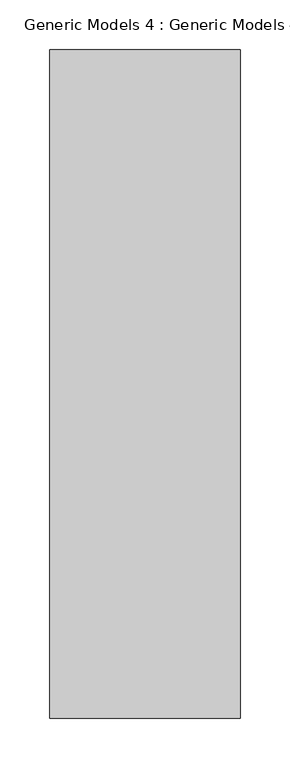
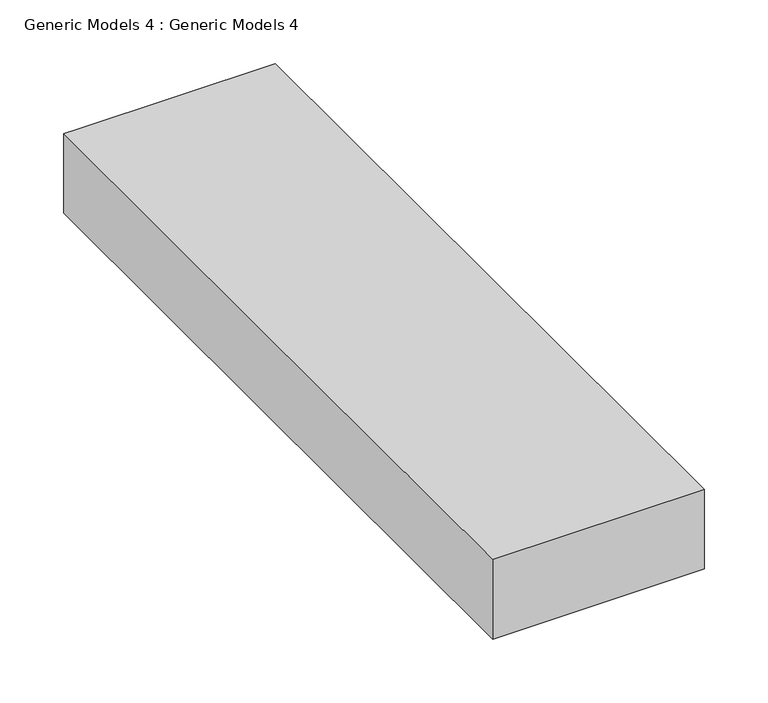
"""IFC4 building model written with IfcOpenShell, lengths in millimetres: proxy geometry, Generic Models 4 : Generic Models 4."""

from ifc_helpers import new_model, si_unit, origin, place, context, project, spatial, faceted_brep, source, transform, mapped, element, save


def generic_models_4_generic_models_4_66c3474a(model_context):
    return source(origin(), model_context, "Body", "Brep", [
        faceted_brep([(-12898.9518575, -15154.7378384, 7008.0330206), (-12898.9518575, -15459.5378384, 7008.0330206), (-12898.9518575, -15827.8378384, 7008.0330206), (-12707.2995814, -15827.8378384, 7008.0330206), (-12707.2995814, -15154.7378384, 7008.0330206), (-12886.2518575, -15154.7378384, 7008.0330206), (-12898.9518575, -15154.7378384, 6931.8330206), (-12886.2518575, -15154.7378384, 6931.8330206), (-12707.2995814, -15154.7378384, 6931.8330206), (-12707.2995814, -15826.0752214, 6931.8330206), (-12707.2995814, -15827.8378384, 6931.8330206), (-12898.9518575, -15827.8378384, 6931.8330206), (-12898.9518575, -15459.5378384, 6931.8330206), (-12898.9518575, -15827.8378384, 6957.2330206), (-12707.2995814, -15827.8378384, 6957.2330206)], [[[0, 1, 2, 3, 4, 5]], [[6, 7, 8, 9, 10, 11, 12]], [[2, 1, 0, 6, 12, 11, 13]], [[3, 2, 13, 11, 10, 14]], [[4, 3, 14, 10, 9, 8]], [[0, 5, 4, 8, 7, 6]]]),
    ])


if __name__ == "__main__":
    model = new_model("IFC4")
    model_context = context("Model", 3, world=origin())
    ifc_project = project(units=[si_unit("LENGTHUNIT", "METRE", prefix="MILLI")], contexts=[model_context])
    site = spatial("IfcSite", under=ifc_project)
    building = spatial("IfcBuilding", under=site)
    placement = place(None, origin())
    generic_models_4_generic_models_4_shape = generic_models_4_generic_models_4_66c3474a(model_context)
    element("IfcBuildingElementProxy", 1, Name="Generic Models 4 : Generic Models 4", ObjectType="Generic Models 4 : Generic Models 4", at=placement, inside=building, context=model_context, shape_type="MappedRepresentation", body=[
        mapped(generic_models_4_generic_models_4_shape, transform((0.0, 0.0, 0.0), x_axis=(1.0, 0.0, 0.0), y_axis=(0.0, 1.0, 0.0), z_axis=(0.0, 0.0, 1.0))),
    ])
    save(model, "model.ifc")
